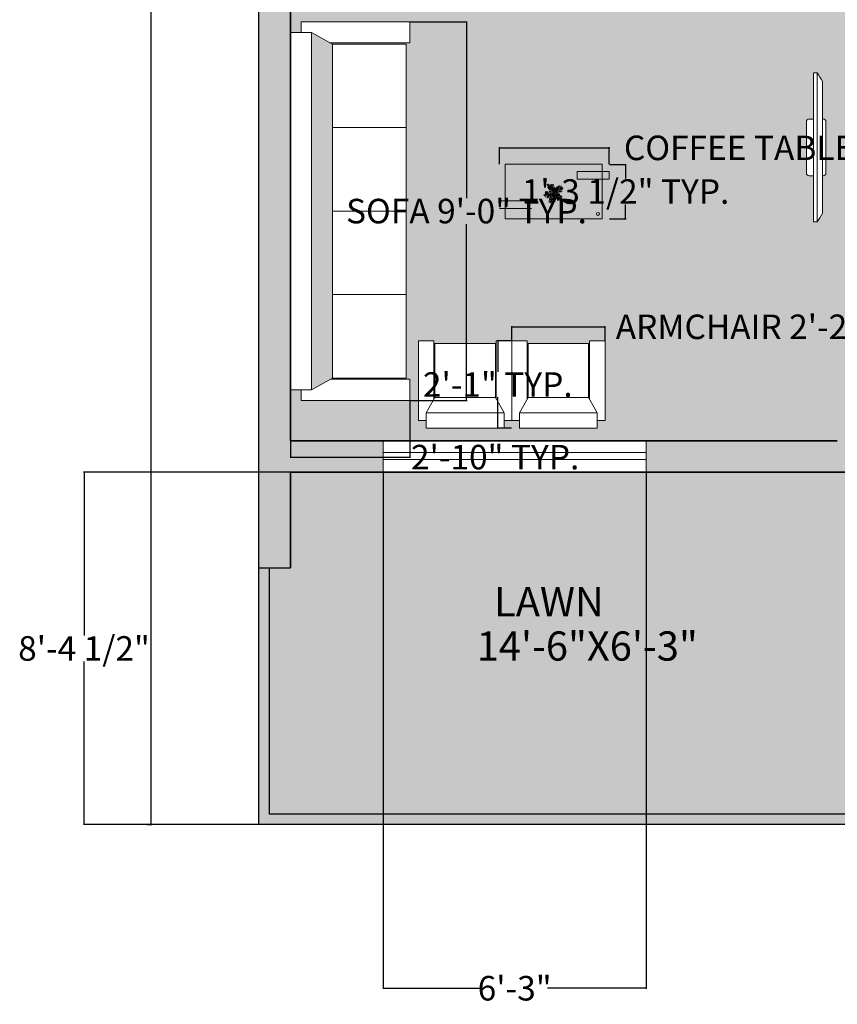
# Model space of a CAD drawing. Units: inches. Extents: x 1884 to 2398, y 474 to 1488.
# Tile 1 of 39: x 1884 to 2118, y 480 to 761. Entities that reach past the tile are written whole.
import ezdxf

# ---------------------------------------------------------------- set-up
doc = ezdxf.new("R2010")
doc.units = ezdxf.units.IN
doc.header["$MEASUREMENT"] = 0
doc.layers.get('0').update_dxf_attribs({"color": 250})
for name, color, linetype, lineweight in [('A-ANNO-DIMS', 2, 'Continuous', 18), ('A-AREA-IDEN', 7, 'Continuous', 18), ('A-EQPM', 8, 'Continuous', 18), ('A-FLOR-PATT', 254, 'Continuous', 13), ('A-FURN-PATT', 253, 'Continuous', 13), ('A-WALL-PATT', 250, 'Continuous', 13), ('C-PROP', 7, 'Continuous', 30), ('furniture', 8, 'Continuous', 18), ('L-PLNT', 73, 'Continuous', 18), ('L-TURF-PATT', 73, 'Continuous', 13), ('walls', 7, 'Continuous', 35), ('windows', 4, 'Continuous', 18)]:
    doc.layers.add(name, color=color, linetype=linetype, lineweight=lineweight)
doc.layers.add('A-FLOR-CASE-PATT', color=251, linetype='Continuous', lineweight=13, true_color=0x636466)
doc.styles.get("Standard").update_dxf_attribs({"font": 'arial.ttf'})
doc.dimstyles.get("Standard").update_dxf_attribs({"dimtxt": 7, "dimasz": 0.18, "dimexe": 0.18, "dimexo": 0.0625, "dimgap": 0.09, "dimtad": 0, "dimtih": 1, "dimtoh": 1, "dimzin": 0, "dimdsep": 46, "dimlunit": 3, "dimtxsty": 'Standard', "dimcen": 0.09, "dimadec": 0, "dimazin": 0, "dimtfac": 1, "dimtofl": 0, "dimtmove": 0, "dimatfit": 3, "dimfxl": 1, "dimtolj": 1, "dimtzin": 0, "dimarcsym": 0})

# ---------------------------------------------------------------- blocks, each defined once
blk = doc.blocks.new('*D2')
at = {"layer": 'A-ANNO-DIMS', "color": 0, "lineweight": -2, "transparency": 16777216}
for p, q in [((1920.51, 1406.88), (1921.96, 1406.88)), ((1921.78, 1406.7), (1921.78, 972.55)), ((1921.78, 531.06), (1921.78, 965.22)), ((1920.51, 530.88), (1921.96, 530.88))]:
    blk.add_line(p, q, dxfattribs=at)
at = {"layer": 'A-ANNO-DIMS', "color": 0, "lineweight": 100, "transparency": 16777216}
for points in [[(1921.75, 1406.7), (1921.81, 1406.7), (1921.78, 1406.88)], [(1921.75, 531.06), (1921.81, 531.06), (1921.78, 530.88)]]:
    blk.add_solid(points, dxfattribs=at)
at = {"layer": 'Defpoints', "color": 0, "lineweight": 100, "transparency": 16777216}
for p in [(1920.45, 1406.88), (1920.45, 530.88), (1921.78, 530.88)]:
    blk.add_point(p, dxfattribs=at)
at = {"layer": 'A-ANNO-DIMS', "color": 0, "transparency": 16777216, "insert": (1921.78, 968.88), "char_height": 7, "attachment_point": 5}
blk.add_mtext("\\A1;73'", dxfattribs=at)
blk = doc.blocks.new('tpoy')
at = {"layer": 'furniture'}
h = blk.add_hatch(color=256, dxfattribs=at)
h.dxf.hatch_style = 1
h.paths.add_polyline_path([(278.09, -251.06), (275.9, -251.06), (275.9, -258.19), (278.09, -258.19)])
h.paths.add_polyline_path([(278.09, -249.1), (275.9, -249.1), (275.9, -251.06), (278.09, -251.06)])
h.paths.add_polyline_path([(286.44, -271.28), (284.25, -271.28), (284.25, -278.76), (286.44, -278.76)])
h.paths.add_polyline_path([(286.44, -278.76), (284.25, -278.76), (284.25, -280.38), (286.44, -280.38)])
for p, q in [((275.9, -249.1), (278.09, -249.1)), ((275.9, -258.19), (275.9, -249.1)), ((278.09, -249.1), (278.09, -258.19)), ((273.86, -251.06), (273.86, -278.76)), ((289.38, -251.06), (273.86, -251.06)), ((289.38, -278.76), (289.38, -251.06)), ((278.09, -258.19), (275.9, -258.19)), ((284.25, -280.38), (284.25, -271.28)), ((286.44, -271.28), (286.44, -280.38)), ((273.86, -278.76), (289.38, -278.76))]:
    blk.add_line(p, q, dxfattribs=at)
blk.add_circle((288.03, -252.28), 0.401, dxfattribs=at)
blk = doc.blocks.new('*U20')
for p, q in [((-10.186, 53.64), (-13.084, 55.962)), ((0, 0), (-10.5, 57)), ((-9.099, 51.782), (-6.563, 55.962)), ((-47.498, 19.737), (-55.83, 18.344)), ((-40.615, 13.7), (-55.105, 10.913)), ((-31.5, 4.5), (-52.5, 25.5)), ((-33.37, 6.269), (-52.207, 5.34)), ((-48.585, 21.131), (-49.309, 29.026)), ((-28.299, 3.483), (-47.86, -5.805)), ((-43.513, 28.561), (-42.427, 15.558)), ((-38.442, 26.239), (-34.819, 7.663)), ((-21.416, 3.018), (-38.079, -8.128)), ((-35.544, 28.097), (-24.314, 3.947)), ((0, 0), (-31.5, 4.5)), ((-14.533, 2.09), (-30.834, 25.31)), ((-15.982, 2.09), (-30.11, -9.521)), ((-3.665, 19.273), (-27.574, 35.527)), ((-5.114, 28.097), (-24.676, 40.636)), ((-24.314, 23.917), (-2.941, 13.7)), ((0, 0), (-22.5, -19.5)), ((-7.288, 39.707), (-21.778, 46.673)), ((-6.563, 1.161), (-21.416, -8.128)), ((-20.691, 13.7), (-1.129, 4.876)), ((-8.737, 47.138), (-17.069, 52.711)), ((-7.65, 43.423), (-2.578, 49.46)), ((-5.839, 35.992), (4.667, 48.067)), ((-5.114, 27.632), (10.463, 46.673)), ((-2.941, 16.486), (8.652, 37.85)), ((-1.129, 6.734), (9.014, 26.704)), ((0, 0), (27, 9)), ((0, 0), (18, -22.5)), ((3.942, 1.625), (11.187, 24.381)), ((6.478, 1.625), (26.04, -8.592)), ((10.101, 3.483), (17.708, 26.239)), ((11.187, 3.483), (30.749, -5.805)), ((16.259, 5.805), (23.142, 31.348)), ((18.07, 5.805), (35.096, -3.483)), ((22.055, 7.198), (27.489, 32.277)), ((24.229, 7.663), (46.688, 1.625)), ((27, 9), (48, 36)), ((27.127, 9.056), (31.112, 35.992)), ((29.662, 12.307), (48.137, 6.269)), ((31.836, 30.883), (32.561, 16.486)), ((33.285, 16.486), (48.862, 10.913)), ((35.096, 32.741), (37.27, 22.524)), ((36.183, 19.737), (48.137, 17.88)), ((38.719, 34.134), (41.979, 28.561)), ((40.53, 25.775), (48.862, 24.846)), ((43.791, 29.954), (51.036, 30.883)), ((44.153, 36.456), (45.239, 32.741)), ((-17.431, -15.094), (-42.789, -18.809)), ((-28.299, -29.026), (-42.789, -31.348)), ((-24.314, -21.596), (-42.427, -22.06)), ((-30.834, -34.135), (-42.427, -35.528)), ((-34.457, -39.708), (-40.978, -42.494)), ((-26.849, -26.24), (-40.253, -25.775)), ((-22.5, -19.5), (-37.5, -45)), ((-32.646, -36.921), (-31.921, -44.352)), ((-15.257, -12.772), (-30.11, -12.772)), ((-29.023, -30.884), (-27.936, -43.887)), ((-25.038, -23.918), (-22.865, -45.281)), ((-20.691, -18.345), (-17.793, -44.352)), ((-6.563, -5.805), (-19.967, -9.985)), ((-17.069, -15.094), (-12.721, -40.172)), ((-13.446, -11.378), (-8.737, -32.741)), ((-9.461, -8.592), (-6.201, -23.453)), ((-4.752, -3.483), (-3.665, -14.629)), ((2.493, -3.019), (-1.491, -20.202)), ((1.769, -2.555), (24.229, -9.521)), ((5.029, -6.27), (2.131, -25.775)), ((9.014, -11.378), (3.58, -35.992)), ((14.085, -16.951), (6.478, -40.172)), ((7.565, -9.056), (32.198, -14.629)), ((18.07, -22.524), (8.289, -45.745)), ((12.274, -15.094), (36.907, -18.809)), ((20.244, -30.419), (15.897, -44.816)), ((16.259, -19.738), (36.183, -22.989)), ((18, -22.5), (27, -52.5)), ((18.433, -22.524), (40.53, -29.026)), ((19.157, -25.311), (38.719, -33.206)), ((22.78, -37.85), (19.519, -48.532)), ((21.331, -32.741), (39.081, -40.636)), ((22.78, -38.314), (34.372, -44.816)), ((24.591, -45.745), (23.142, -50.854)), ((24.591, -43.423), (30.749, -47.603)), ((26.764, -49.925), (28.213, -50.854))]:
    blk.add_line(p, q)
blk = doc.blocks.new('PLASMA-LARGE')
at = {"layer": 'furniture'}
for p, q in [((-7.26, 0), (7.26, 0)), ((-21, -2.5), (21, -2.5)), ((-21, -2.5), (-21, -3.5)), ((-18.61, -1), (18.61, -1)), ((-8, -1), (-8, -0.74)), ((8, -1), (8, -0.74)), ((21, -2.5), (21, -3.5)), ((-21, -3.5), (21, -3.5)), ((-8, -3.5), (-8, -4.76)), ((-7.26, -5.5), (7.26, -5.5)), ((8, -3.5), (8, -4.76))]:
    blk.add_line(p, q, dxfattribs=at)
for centre, radius, start, end in [((-7.26, -0.74), 0.744, 90, 180), ((7.26, -0.74), 0.744, 0, 90), ((-13.97, -11.05), 11.07, 114.7602, 129.4175), ((13.97, -11.05), 11.07, 50.5825, 65.2398), ((-7.26, -4.76), 0.744, 180, 270), ((7.26, -4.76), 0.744, 270, 0)]:
    blk.add_arc(centre, radius, start, end, dxfattribs=at)
blk = doc.blocks.new('FABRIC SOFA 4S')
at = {"layer": 'furniture'}
for p, q in [((3, 54), (34, 54)), ((3, 51), (3, 54)), ((34, 48), (34, 54)), ((0, -51), (0, 51)), ((6, 51), (0, 51)), ((6, -51), (6, 51)), ((12, 47.63), (6, 51)), ((11.14, 48), (34, 48)), ((33, 23.81), (12, 23.81)), ((33, 0), (12, 0)), ((33, -23.81), (12, -23.81)), ((6, -51), (12, -47.63)), ((11.54, -48), (34, -48)), ((34, -48), (34, -54)), ((6, -51), (0, -51)), ((3, -54), (3, -51)), ((3, -54), (34, -54))]:
    blk.add_line(p, q, dxfattribs=at)
blk.add_lwpolyline([(12, -47.63), (12, 47.63), (33, 47.63), (33, -47.63)], close=True, dxfattribs=at)
blk = doc.blocks.new('FABRIC SOFA 1S')
at = {"layer": 'furniture'}
for p, q in [((3, 18.12), (34, 18.12)), ((3, 15.12), (3, 18.12)), ((34, 12.12), (34, 18.12)), ((0, -15.12), (0, 15.12)), ((6, 15.12), (0, 15.12)), ((6, -15.12), (6, 15.12)), ((12, 11.75), (6, 15.12)), ((11.33, 12.12), (34, 12.12)), ((6, -15.12), (0, -15.12)), ((3, -18.12), (3, -15.12)), ((6, -15.12), (12, -11.75)), ((11.33, -12.12), (34, -12.12)), ((34, -12.12), (34, -18.12)), ((3, -18.12), (34, -18.12))]:
    blk.add_line(p, q, dxfattribs=at)
blk.add_lwpolyline([(12, -11.75), (12, 11.75), (33, 11.75), (33, -11.75)], close=True, dxfattribs=at)
blk = doc.blocks.new('*D29')
at = {"layer": 'A-ANNO-DIMS', "color": 0, "lineweight": -2, "transparency": 16777216}
for p, q in [((2024.65, 668.97), (2024.65, 673.08)), ((2024.83, 672.9), (2051.08, 672.9)), ((2051.26, 668.97), (2051.26, 673.08)), ((2051.26, 672.9), (2051.44, 672.9))]:
    blk.add_line(p, q, dxfattribs=at)
at = {"layer": 'A-ANNO-DIMS', "color": 0, "lineweight": 100, "transparency": 16777216}
for points in [[(2024.83, 672.93), (2024.83, 672.87), (2024.65, 672.9)], [(2051.08, 672.93), (2051.08, 672.87), (2051.26, 672.9)]]:
    blk.add_solid(points, dxfattribs=at)
at = {"layer": 'Defpoints', "color": 0, "lineweight": 100, "transparency": 16777216}
for p in [(2051.26, 672.9), (2024.65, 668.91), (2051.26, 668.91)]:
    blk.add_point(p, dxfattribs=at)
at = {"layer": 'A-ANNO-DIMS', "color": 0, "transparency": 16777216, "insert": (2108.66, 672.9), "char_height": 7, "attachment_point": 5}
blk.add_mtext('\\A1;ARMCHAIR 2\'-2 1/2" TYP.', dxfattribs=at)
blk = doc.blocks.new('*D30')
at = {"layer": 'A-ANNO-DIMS', "color": 0, "lineweight": -2, "transparency": 16777216}
for p, q in [((2024.59, 668.91), (2020.48, 668.91)), ((2020.66, 668.73), (2020.66, 660.04)), ((2020.66, 644.14), (2020.66, 652.83)), ((2024.59, 643.96), (2020.48, 643.96))]:
    blk.add_line(p, q, dxfattribs=at)
at = {"layer": 'A-ANNO-DIMS', "color": 0, "lineweight": 100, "transparency": 16777216}
for points in [[(2020.63, 668.73), (2020.69, 668.73), (2020.66, 668.91)], [(2020.63, 644.14), (2020.69, 644.14), (2020.66, 643.96)]]:
    blk.add_solid(points, dxfattribs=at)
at = {"layer": 'Defpoints', "color": 0, "lineweight": 100, "transparency": 16777216}
for p in [(2020.66, 668.91), (2024.65, 668.91), (2024.65, 643.96)]:
    blk.add_point(p, dxfattribs=at)
at = {"layer": 'A-ANNO-DIMS', "color": 0, "transparency": 16777216, "insert": (2020.66, 656.43), "char_height": 7, "attachment_point": 5}
blk.add_mtext('\\A1;2\'-1" TYP.', dxfattribs=at)
blk = doc.blocks.new('*D31')
at = {"layer": 'A-ANNO-DIMS', "color": 0, "lineweight": -2, "transparency": 16777216}
for p, q in [((1995.59, 759.92), (2011.91, 759.92)), ((2011.73, 759.74), (2011.73, 709.63)), ((2011.73, 652.1), (2011.73, 702.2)), ((1995.59, 651.92), (2011.91, 651.92))]:
    blk.add_line(p, q, dxfattribs=at)
at = {"layer": 'A-ANNO-DIMS', "color": 0, "lineweight": 100, "transparency": 16777216}
for points in [[(2011.7, 759.74), (2011.76, 759.74), (2011.73, 759.92)], [(2011.7, 652.1), (2011.76, 652.1), (2011.73, 651.92)]]:
    blk.add_solid(points, dxfattribs=at)
at = {"layer": 'Defpoints', "color": 0, "lineweight": 100, "transparency": 16777216}
for p in [(1995.53, 759.92), (2011.73, 759.92), (1995.53, 651.92)]:
    blk.add_point(p, dxfattribs=at)
at = {"layer": 'A-ANNO-DIMS', "color": 0, "transparency": 16777216, "insert": (2011.73, 705.92), "char_height": 7, "attachment_point": 5}
blk.add_mtext('\\A1;SOFA 9\'-0" TYP.', dxfattribs=at)
blk = doc.blocks.new('*D32')
at = {"layer": 'A-ANNO-DIMS', "color": 0, "lineweight": -2, "transparency": 16777216}
for p, q in [((1961.53, 651.85), (1961.53, 635.54)), ((1995.53, 651.85), (1995.53, 635.54)), ((1961.71, 635.72), (1995.35, 635.72)), ((1995.53, 635.72), (1995.71, 635.72))]:
    blk.add_line(p, q, dxfattribs=at)
at = {"layer": 'A-ANNO-DIMS', "color": 0, "lineweight": 100, "transparency": 16777216}
for points in [[(1961.71, 635.75), (1961.71, 635.69), (1961.53, 635.72)], [(1995.35, 635.75), (1995.35, 635.69), (1995.53, 635.72)]]:
    blk.add_solid(points, dxfattribs=at)
at = {"layer": 'Defpoints', "color": 0, "lineweight": 100, "transparency": 16777216}
for p in [(1961.53, 651.92), (1995.53, 651.92), (1995.53, 635.72)]:
    blk.add_point(p, dxfattribs=at)
at = {"layer": 'A-ANNO-DIMS', "color": 0, "transparency": 16777216, "insert": (2019.91, 635.72), "char_height": 7, "attachment_point": 5}
blk.add_mtext('\\A1;2\'-10" TYP.', dxfattribs=at)
blk = doc.blocks.new('*D33')
at = {"layer": 'A-ANNO-DIMS', "color": 0, "lineweight": -2, "transparency": 16777216}
for p, q in [((2021.15, 719.33), (2021.15, 724.14)), ((2021.33, 723.96), (2052.25, 723.96)), ((2052.43, 719.33), (2052.43, 724.14)), ((2052.43, 723.96), (2052.61, 723.96))]:
    blk.add_line(p, q, dxfattribs=at)
at = {"layer": 'A-ANNO-DIMS', "color": 0, "lineweight": 100, "transparency": 16777216}
for points in [[(2021.33, 723.99), (2021.33, 723.93), (2021.15, 723.96)], [(2052.25, 723.99), (2052.25, 723.93), (2052.43, 723.96)]]:
    blk.add_solid(points, dxfattribs=at)
at = {"layer": 'Defpoints', "color": 0, "lineweight": 100, "transparency": 16777216}
for p in [(2052.43, 723.96), (2021.15, 719.26), (2052.43, 719.26)]:
    blk.add_point(p, dxfattribs=at)
at = {"layer": 'A-ANNO-DIMS', "color": 0, "transparency": 16777216, "insert": (2120.18, 723.96), "char_height": 7, "attachment_point": 5}
blk.add_mtext('\\A1;COFFEE TABLE 2\'-7 1/2" TYP.', dxfattribs=at)
blk = doc.blocks.new('*D34')
at = {"layer": 'A-ANNO-DIMS', "color": 0, "lineweight": -2, "transparency": 16777216}
for p, q in [((2052.49, 719.26), (2057.3, 719.26)), ((2057.12, 719.08), (2057.12, 715.21)), ((2057.12, 703.92), (2057.12, 707.79)), ((2052.49, 703.74), (2057.3, 703.74))]:
    blk.add_line(p, q, dxfattribs=at)
at = {"layer": 'A-ANNO-DIMS', "color": 0, "lineweight": 100, "transparency": 16777216}
for points in [[(2057.09, 719.08), (2057.15, 719.08), (2057.12, 719.26)], [(2057.09, 703.92), (2057.15, 703.92), (2057.12, 703.74)]]:
    blk.add_solid(points, dxfattribs=at)
at = {"layer": 'Defpoints', "color": 0, "lineweight": 100, "transparency": 16777216}
for p in [(2052.43, 719.26), (2052.43, 703.74), (2057.12, 703.74)]:
    blk.add_point(p, dxfattribs=at)
at = {"layer": 'A-ANNO-DIMS', "color": 0, "transparency": 16777216, "insert": (2057.12, 711.5), "char_height": 7, "attachment_point": 5}
blk.add_mtext('\\A1;1\'-3 1/2" TYP.', dxfattribs=at)
blk = doc.blocks.new('*D55')
at = {"layer": 'A-ANNO-DIMS', "color": 0, "lineweight": -2, "transparency": 16777216}
for p, q in [((1988, 631.32), (1988, 484)), ((2062.95, 631.32), (2062.95, 484)), ((1988.18, 484.18), (2016.06, 484.18)), ((2062.77, 484.18), (2034.89, 484.18))]:
    blk.add_line(p, q, dxfattribs=at)
at = {"layer": 'A-ANNO-DIMS', "color": 0, "lineweight": 100, "transparency": 16777216}
for points in [[(1988.18, 484.21), (1988.18, 484.15), (1988, 484.18)], [(2062.77, 484.21), (2062.77, 484.15), (2062.95, 484.18)]]:
    blk.add_solid(points, dxfattribs=at)
at = {"layer": 'Defpoints', "color": 0, "lineweight": 100, "transparency": 16777216}
for p in [(1988, 631.38), (2062.95, 631.38), (2062.95, 484.18)]:
    blk.add_point(p, dxfattribs=at)
at = {"layer": 'A-ANNO-DIMS', "color": 0, "transparency": 16777216, "insert": (2025.48, 484.18), "char_height": 7, "attachment_point": 5}
blk.add_mtext('\\A1;6\'-3"', dxfattribs=at)
blk = doc.blocks.new('*D56')
at = {"layer": 'A-ANNO-DIMS', "color": 0, "lineweight": -2, "transparency": 16777216}
for p, q in [((1961.47, 631.38), (1902.43, 631.38)), ((1902.61, 631.2), (1902.61, 584.84)), ((1902.61, 531.06), (1902.61, 577.43)), ((1952.47, 530.88), (1902.43, 530.88))]:
    blk.add_line(p, q, dxfattribs=at)
at = {"layer": 'A-ANNO-DIMS', "color": 0, "lineweight": 100, "transparency": 16777216}
for points in [[(1902.58, 631.2), (1902.64, 631.2), (1902.61, 631.38)], [(1902.58, 531.06), (1902.64, 531.06), (1902.61, 530.88)]]:
    blk.add_solid(points, dxfattribs=at)
at = {"layer": 'Defpoints', "color": 0, "lineweight": 100, "transparency": 16777216}
for p in [(1902.61, 631.38), (1961.53, 631.38), (1952.53, 530.88)]:
    blk.add_point(p, dxfattribs=at)
at = {"layer": 'A-ANNO-DIMS', "color": 0, "transparency": 16777216, "insert": (1902.61, 581.13), "char_height": 7, "attachment_point": 5}
blk.add_mtext('\\A1;8\'-4 1/2"', dxfattribs=at)

msp = doc.modelspace()

# ---------------------------------------------------------------- hatches: boundary and pattern name
at = {"layer": 'A-FLOR-CASE-PATT'}
h = msp.add_hatch(color=256, dxfattribs=at)
h.dxf.hatch_style = 1
h.paths.add_polyline_path([(2101.332, 755.284), (2116.228, 755.284), (2116.228, 690.841), (2101.332, 690.841)])
h.paths.add_polyline_path([(2110.739, 702.864), (2111.75, 702.864, 0.0640419), (2113.267, 705.284), (2113.267, 716.011), (2113.526, 716.011, 0.4142136), (2114.278, 716.764), (2114.278, 731.439, 0.4142136), (2113.526, 732.192), (2113.267, 732.192), (2113.267, 742.92, 0.0640419), (2111.75, 745.339), (2110.739, 745.339), (2110.739, 732.192), (2109.469, 732.192, 0.4142136), (2108.716, 731.439), (2108.716, 716.764, 0.4142136), (2109.469, 716.011), (2110.739, 716.011)], flags=16)
at = {"layer": 'A-FLOR-PATT'}
h = msp.add_hatch(color=256, dxfattribs=at)
h.dxf.hatch_style = 1
h.paths.add_polyline_path([(2117.529, 815.801), (2126.529, 815.801), (2126.529, 880.382), (2117.529, 880.382), (2117.529, 892.385), (1961.529, 892.385), (1961.529, 756.915), (1964.529, 756.915), (1964.529, 759.915), (1995.529, 759.915), (1995.529, 753.915), (1972.862, 753.915), (1967.529, 756.915), (1967.529, 654.915), (1972.862, 657.915), (1995.529, 657.915), (1995.529, 651.915), (1964.529, 651.915), (1964.529, 654.915), (1961.529, 654.915), (1961.529, 640.385), (2117.529, 640.385), (2117.529, 646.578), (2126.529, 646.578), (2126.529, 676.183), (2117.529, 676.183)])
h.paths.add_polyline_path([(2012.246, 808.929), (2012.05, 810.185), (2032.542, 810.185), (2032.346, 808.929)], flags=16)
h.paths.add_polyline_path([(2010.381, 820.864), (1994.658, 820.864), (1994.658, 831.561), (1984.608, 833.132), (1984.608, 853.821), (1994.658, 855.391), (1994.658, 866.089), (2010.381, 866.089), (2011.951, 876.139), (2032.64, 876.139), (2034.211, 866.089), (2045.556, 866.089), (2047.127, 876.139), (2067.816, 876.139), (2069.386, 866.089), (2085.109, 866.089), (2085.109, 855.391), (2095.159, 853.821), (2095.159, 833.132), (2085.109, 831.561), (2085.109, 820.864), (2069.386, 820.864), (2067.816, 810.814), (2047.127, 810.814), (2045.556, 820.864), (2034.211, 820.864), (2032.64, 810.814), (2011.951, 810.814)], flags=16)
h.paths.add_polyline_path([(1982.724, 833.426), (1982.724, 853.526), (1983.98, 853.723), (1983.98, 833.23)], flags=16)
h.paths.add_polyline_path([(1994.529, 753.54), (1994.529, 658.29), (1973.529, 658.29), (1973.529, 753.54)], flags=16)
h.paths.add_polyline_path([(2084.486, 843.527), (2084.592, 843.502), (2084.681, 843.487), (2084.813, 843.477), (2084.913, 843.477), (2084.669, 843.482), (2084.336, 843.565), (2084.116, 843.617), (2083.8, 843.686), (2083.105, 843.827), (2082.836, 843.874), (2083.604, 843.729), (2084.206, 843.597)], flags=0)
h.paths.add_polyline_path([(2047.421, 808.929), (2047.225, 810.185), (2067.718, 810.185), (2067.521, 808.929)], flags=16)
h.paths.add_polyline_path([(2066.01, 849.505), (2066.429, 849.687), (2066.798, 849.882), (2067.129, 850.085), (2067.43, 850.293), (2067.711, 850.502), (2068.176, 850.856), (2068.689, 851.205), (2069.305, 851.531), (2070.015, 851.784), (2070.844, 851.944), (2071.081, 851.956), (2070.629, 851.902), (2070.212, 851.822), (2069.827, 851.717), (2069.471, 851.59), (2069.139, 851.443), (2068.828, 851.279), (2068.534, 851.1), (2068.254, 850.909), (2067.983, 850.709), (2067.502, 850.343), (2066.951, 849.962), (2066.224, 849.579)], flags=0)
h.paths.add_polyline_path([(2059.423, 853.221), (2059.827, 853.278), (2060.171, 853.358), (2060.465, 853.463), (2060.714, 853.589), (2060.926, 853.736), (2061.107, 853.902), (2061.258, 854.086), (2061.377, 854.284), (2061.462, 854.495), (2061.514, 854.715), (2061.53, 854.943), (2061.508, 855.176), (2061.449, 855.411), (2061.352, 855.646), (2061.224, 855.882), (2061.07, 856.117), (2060.9, 856.353), (2060.719, 856.588), (2060.406, 856.993), (2060.103, 857.424), (2059.858, 857.888), (2059.691, 858.467), (2059.836, 859.091), (2060.305, 859.532), (2060.844, 859.798), (2061.513, 859.935), (2062.253, 859.905), (2062.483, 859.849), (2062.078, 859.912), (2061.695, 859.928), (2061.336, 859.899), (2061.005, 859.831), (2060.703, 859.729), (2060.437, 859.597), (2060.208, 859.441), (2060.021, 859.265), (2059.879, 859.075), (2059.785, 858.874), (2059.737, 858.664), (2059.73, 858.447), (2059.761, 858.224), (2059.827, 857.996), (2059.923, 857.765), (2060.047, 857.53), (2060.193, 857.295), (2060.359, 857.06), (2060.537, 856.824), (2060.867, 856.399), (2061.171, 855.978), (2061.422, 855.518), (2061.567, 854.943), (2061.41, 854.272), (2060.947, 853.707), (2060.335, 853.397), (2059.649, 853.236)], flags=0)
h.paths.add_polyline_path([(2050.778, 859.745), (2051.07, 859.87), (2051.295, 860.017), (2051.467, 860.183), (2051.594, 860.365), (2051.679, 860.56), (2051.726, 860.763), (2051.739, 860.971), (2051.722, 861.18), (2051.677, 861.387), (2051.609, 861.587), (2051.521, 861.779), (2051.421, 861.962), (2051.312, 862.138), (2051.203, 862.307), (2050.966, 862.68), (2050.793, 863.193), (2051.021, 863.699), (2051.483, 864.018), (2052.09, 864.138), (2052.773, 864.157), (2053.007, 864.142), (2052.603, 864.152), (2052.258, 864.142), (2051.965, 864.113), (2051.716, 864.064), (2051.504, 863.995), (2051.322, 863.907), (2051.17, 863.802), (2051.048, 863.682), (2050.954, 863.55), (2050.891, 863.408), (2050.856, 863.259), (2050.851, 863.105), (2050.876, 862.948), (2050.929, 862.791), (2051.005, 862.633), (2051.098, 862.472), (2051.203, 862.307), (2051.312, 862.138), (2051.556, 861.742), (2051.751, 861.167), (2051.712, 860.535), (2051.398, 860.085), (2050.949, 859.79)], flags=0)
h.paths.add_polyline_path([(2022.768, 719.264), (2050.461, 719.264), (2050.461, 717.226), (2052.426, 717.226), (2052.426, 715.033), (2050.461, 715.033), (2050.461, 703.738), (2022.768, 703.738)], flags=16)
h.paths.add_polyline_path([(2012.246, 878.023), (2032.346, 878.023), (2032.542, 876.767), (2012.05, 876.767)], flags=16)
h.paths.add_polyline_path([(2035.324, 713.103), (2035.342, 713.294), (2035.192, 713.202)], flags=0)
h.paths.add_polyline_path([(2036.484, 711.63), (2036.583, 711.849), (2036.39, 711.898)], flags=0)
h.paths.add_polyline_path([(2036.074, 712.744), (2035.993, 712.481), (2035.724, 712.516), (2035.794, 712.726)], flags=0)
h.paths.add_polyline_path([(2035.846, 710.909), (2035.753, 710.958), (2035.702, 710.88)], flags=0)
h.paths.add_polyline_path([(2037.818, 712.019), (2037.948, 712.06), (2037.987, 712.161), (2037.815, 712.02)], flags=0)
h.paths.add_polyline_path([(2038.451, 709.517), (2038.464, 709.428), (2038.586, 709.442)], flags=0)
h.paths.add_polyline_path([(2037.805, 709.806), (2037.818, 709.807), (2037.804, 709.823)], flags=0)
h.paths.add_polyline_path([(2036.7, 711.245), (2036.698, 711.236), (2036.813, 711.211)], flags=0)
h.paths.add_polyline_path([(2035.928, 708.897), (2035.668, 708.871), (2035.706, 708.667)], flags=0)
h.paths.add_polyline_path([(2036.414, 710.976), (2035.932, 709.859), (2036.792, 710.484), (2036.5, 710.934)], flags=0)
h.paths.add_polyline_path([(2038.298, 712.115), (2038.499, 712.058), (2038.612, 712.269), (2038.39, 712.332)], flags=0)
h.paths.add_polyline_path([(2047.421, 878.023), (2067.521, 878.023), (2067.718, 876.767), (2047.225, 876.767)], flags=16)
h.paths.add_polyline_path([(2049.647, 705.093, -1), (2048.845, 705.093, -1)], flags=0)
h.paths.add_polyline_path([(2095.787, 853.723), (2097.043, 853.526), (2097.043, 833.426), (2095.787, 833.23)], flags=16)
h.paths.add_polyline_path([(2110.739, 745.339), (2111.75, 745.339, -0.0640419), (2113.267, 742.92), (2113.267, 732.192), (2113.526, 732.192, -0.4142136), (2114.278, 731.439), (2114.278, 716.764, -0.4142136), (2113.526, 716.011), (2113.267, 716.011), (2113.267, 705.284, -0.0640419), (2111.75, 702.864), (2110.739, 702.864), (2110.739, 716.011), (2109.469, 716.011, -0.4142136), (2108.716, 716.764), (2108.716, 731.439, -0.4142136), (2109.469, 732.192), (2110.739, 732.192)], flags=16)
h.paths.add_polyline_path([(1998.045, 668.909), (2002.449, 668.909), (2002.449, 652.273), (2002.724, 652.763), (2002.724, 668.175), (2019.972, 668.175), (2019.972, 652.763), (2020.247, 652.273), (2020.247, 668.909), (2024.651, 668.909), (2029.055, 668.909), (2029.055, 652.273), (2029.33, 652.763), (2029.33, 668.175), (2046.578, 668.175), (2046.578, 652.763), (2046.853, 652.273), (2046.853, 668.909), (2051.257, 668.909), (2051.257, 646.157), (2049.055, 646.157), (2049.055, 643.955), (2026.853, 643.955), (2026.853, 646.157), (2024.651, 646.157), (2022.449, 646.157), (2022.449, 643.955), (2000.247, 643.955), (2000.247, 646.157), (1998.045, 646.157)], flags=16)
h.paths.add_polyline_path([(2342.529, 1247.885), (2265.892, 1247.885), (2230.029, 1247.885), (2209.755, 1247.885), (2168.6, 1247.885), (2168.6, 1104.929), (2158.029, 1104.929), (2158.029, 1079.411), (2168.6, 1079.411), (2168.6, 1062.466), (2342.529, 1062.466), (2342.529, 1093.809)])
h.paths.add_polyline_path([(2215.03, 1153.876), (2215.03, 1164.739), (2187.559, 1164.739), (2187.442, 1152.641), (2173.568, 1152.641), (2173.684, 1164.739), (2173.684, 1218.739), (2173.801, 1230.837), (2187.675, 1230.837), (2187.559, 1218.739), (2215.03, 1218.739), (2215.03, 1225.879), (2245.053, 1225.879), (2245.053, 1153.876)], flags=16)
h.paths.add_polyline_path([(2192.147, 1164.797), (2184.963, 1174.54), (2184.915, 1174.54), (2176.755, 1174.54), (2176.755, 1190.363), (2184.915, 1190.363), (2184.915, 1196.819), (2176.755, 1196.819), (2176.755, 1212.641), (2184.915, 1212.641), (2184.915, 1174.606), (2184.963, 1174.54), (2192.147, 1174.54)], flags=0)
h.paths.add_polyline_path([(2184.971, 1158.364, -1), (2176.039, 1158.364, -1)], flags=0)
h.paths.add_polyline_path([(2335.555, 1161.985), (2335.555, 1175.132), (2334.285, 1175.132, -0.4142136), (2333.533, 1175.885), (2333.533, 1190.56, -0.4142136), (2334.285, 1191.313), (2335.555, 1191.313), (2335.555, 1204.46), (2336.567, 1204.46, -0.0640419), (2338.083, 1202.04), (2338.083, 1191.313), (2338.342, 1191.313, -0.4142136), (2339.095, 1190.56), (2339.095, 1175.885, -0.4142136), (2338.342, 1175.132), (2338.083, 1175.132), (2338.083, 1164.405, -0.0640419), (2336.567, 1161.985)], flags=16)
h.paths.add_polyline_path([(2176.155, 1224.462, -1), (2185.087, 1224.462, -1)], flags=0)
h.paths.add_polyline_path([(2158.029, 1276.197), (2158.029, 1322.885), (2148.233, 1322.885), (2092.029, 1322.885), (1961.529, 1322.885), (1961.529, 1166.885), (2116.005, 1166.885), (2116.005, 1157.885), (2152.638, 1157.885), (2152.638, 1166.885), (2158.029, 1166.885)])
h.paths.add_polyline_path([(2006.352, 1204.245), (2006.352, 1215.108), (1978.881, 1215.108), (1978.764, 1203.01), (1964.89, 1203.01), (1965.006, 1215.108), (1965.006, 1269.108), (1965.123, 1281.207), (1978.997, 1281.207), (1978.881, 1269.108), (2006.352, 1269.108), (2006.352, 1276.248), (2036.375, 1276.248), (2036.375, 1204.245)], flags=16)
h.paths.add_polyline_path([(1983.469, 1215.166), (1976.285, 1224.909), (1976.237, 1224.909), (1968.077, 1224.909), (1968.077, 1240.732), (1976.237, 1240.732), (1976.237, 1247.188), (1968.077, 1247.188), (1968.077, 1263.011), (1976.237, 1263.011), (1976.237, 1224.975), (1976.285, 1224.909), (1983.469, 1224.909)], flags=0)
h.paths.add_polyline_path([(1976.293, 1208.733, -1), (1967.361, 1208.733, -1)], flags=0)
h.paths.add_polyline_path([(1967.477, 1274.832, -1), (1976.41, 1274.832, -1)], flags=0)
h.paths.add_polyline_path([(2152.587, 1223.485), (2152.587, 1236.632), (2151.317, 1236.632, -0.4142136), (2150.564, 1237.385), (2150.564, 1252.06, -0.4142136), (2151.317, 1252.813), (2152.587, 1252.813), (2152.587, 1265.959), (2153.598, 1265.959, -0.0640419), (2155.115, 1263.54), (2155.115, 1252.813), (2155.374, 1252.813, -0.4142136), (2156.126, 1252.06), (2156.126, 1237.385, -0.4142136), (2155.374, 1236.632), (2155.115, 1236.632), (2155.115, 1225.904, -0.0640419), (2153.598, 1223.485)], flags=16)
h.paths.add_polyline_path([(2250.676, 1161.101), (2322.077, 1161.101), (2322.077, 1173.886), (2250.676, 1173.886)], flags=24)
h.paths.add_polyline_path([(2255.61, 1173.712), (2320.136, 1173.712), (2320.136, 1186.659), (2255.61, 1186.659)], flags=24)
h.paths.add_polyline_path([(2053.687, 1230.837), (2125.089, 1230.837), (2125.089, 1243.622), (2053.687, 1243.622)], flags=24)
h.paths.add_polyline_path([(2058.622, 1243.448), (2123.147, 1243.448), (2123.147, 1256.395), (2058.622, 1256.395)], flags=24)
at = {"layer": 'A-FURN-PATT'}
h = msp.add_hatch(color=256, dxfattribs=at)
h.dxf.hatch_style = 1
h.paths.add_polyline_path([(2050.461, 715.033), (2043.335, 715.033), (2043.335, 717.226), (2050.461, 717.226), (2050.461, 719.264), (2022.768, 719.264), (2022.768, 708.874), (2030.239, 708.874), (2030.239, 706.68), (2022.768, 706.68), (2022.768, 703.738), (2050.461, 703.738)])
h.paths.add_polyline_path([(2038.607, 712.27), (2038.612, 712.269), (2038.615, 712.273)], flags=16)
h.paths.add_polyline_path([(2036.679, 711.078), (2035.246, 710.788), (2035.256, 710.805), (2035.27, 710.793), (2036.679, 711.078), (2036.195, 712.449), (2036.185, 712.456), (2036.193, 712.455), (2036.679, 711.078), (2036.813, 711.189), (2036.819, 711.21), (2036.835, 711.207), (2036.679, 711.078), (2037.451, 710.216), (2037.462, 710.218), (2037.465, 710.201)], flags=16)
h.paths.add_polyline_path([(2049.647, 705.093, -1), (2048.845, 705.093, -1)], flags=16)
at = {"layer": 'A-WALL-PATT'}
h = msp.add_hatch(color=256, dxfattribs=at)
h.dxf.hatch_style = 1
h.paths.add_polyline_path([(2351.529, 837.963), (2342.529, 837.963), (2342.529, 813.478), (2351.529, 813.478)])
h.paths.add_polyline_path([(2351.529, 782.175), (2342.529, 782.175), (2342.529, 778.966), (2238.447, 778.966), (2238.447, 769.966), (2351.529, 769.966)])
h.paths.add_polyline_path([(2351.529, 914.773), (2342.529, 914.773), (2342.529, 901.966), (2222.529, 901.966), (2222.529, 908.236), (2213.529, 908.236), (2213.529, 901.966), (2198.529, 901.966), (2198.529, 892.966), (2198.529, 815.857), (2203.029, 815.857), (2203.029, 892.966), (2342.529, 892.966), (2342.529, 869.555), (2346.047, 869.555), (2351.529, 869.555), (2351.529, 880.385)])
h.paths.add_polyline_path([(2208.948, 778.966), (2203.029, 778.966), (2203.029, 782.647), (2198.529, 782.647), (2198.529, 779.109), (2193.526, 779.109), (2193.526, 769.966), (2198.529, 769.966), (2208.948, 769.966)])
h.paths.add_polyline_path([(2126.529, 815.801), (2117.529, 815.801), (2117.529, 676.183), (2126.529, 676.183), (2126.529, 769.966), (2132.515, 769.966), (2132.515, 778.664), (2126.529, 778.664)])
h.paths.add_polyline_path([(2135.996, 901.385), (2009.529, 901.385), (2009.529, 929.544), (2000.529, 929.544), (2000.529, 892.385), (2117.529, 892.385), (2117.529, 880.382), (2126.529, 880.382), (2126.529, 892.385), (2135.996, 892.385)])
h.paths.add_polyline_path([(2198.529, 901.385), (2185.2, 901.385), (2185.2, 892.385), (2198.529, 892.385), (2198.529, 892.966)])
h.paths.add_polyline_path([(1961.529, 892.385), (1965.143, 892.385), (1965.143, 901.385), (1952.529, 901.385), (1952.529, 604.13), (1961.529, 604.13), (1961.529, 631.385), (1988.002, 631.385), (1988.002, 640.385), (1961.529, 640.385)])
h.paths.add_polyline_path([(1955.529, 604.13), (1952.529, 604.13), (1952.529, 530.885), (2126.529, 530.885), (2126.529, 533.885), (1955.529, 533.885)])
h.paths.add_polyline_path([(2396.529, 604.13), (2393.529, 604.13), (2393.529, 533.885), (2126.529, 533.885), (2126.529, 530.885), (2396.529, 530.885)])
h.paths.add_polyline_path([(2396.529, 779.322), (2387.529, 779.322), (2387.529, 604.13), (2396.529, 604.13)])
h = msp.add_hatch(color=256, dxfattribs=at)
h.dxf.hatch_style = 1
h.paths.add_polyline_path([(2126.529, 646.578), (2117.529, 646.578), (2117.529, 640.385), (2062.952, 640.385), (2062.952, 631.385), (2126.529, 631.385)])
at = {"layer": 'L-TURF-PATT'}
h = msp.add_hatch(color=256, dxfattribs=at)
h.dxf.hatch_style = 1
h.paths.add_polyline_path([(2126.529, 607.943), (2117.364, 607.943), (2117.364, 631.385), (1961.529, 631.385), (1961.529, 604.13), (1955.529, 604.13), (1955.529, 533.885), (2126.529, 533.885)])
h = msp.add_hatch(color=256, dxfattribs=at)
h.dxf.hatch_style = 1
h.paths.add_polyline_path([(2120.392, 631.385), (2117.364, 631.385), (2117.364, 607.943), (2126.529, 607.943), (2126.529, 611.008), (2120.392, 611.008)])
h.paths.add_polyline_path([(2126.529, 631.385), (2120.392, 631.385), (2120.392, 611.008), (2126.529, 611.008)], flags=17)

# ---------------------------------------------------------------- linework, layer by layer
at = {"layer": 'C-PROP'}
for p, q in [((1952.529, 530.885), (1952.529, 901.385)), ((1952.529, 604.13), (1961.529, 604.13)), ((1955.529, 533.885), (1955.529, 604.13)), ((2393.529, 533.885), (1955.529, 533.885)), ((2396.529, 530.885), (1952.529, 530.885))]:
    msp.add_line(p, q, dxfattribs=at)
at = {"layer": 'walls'}
for p, q in [((1961.529, 640.385), (1961.529, 892.385)), ((1961.529, 640.385), (2117.529, 640.385)), ((1961.529, 604.13), (1961.529, 631.385)), ((1961.529, 631.385), (2126.529, 631.385))]:
    msp.add_line(p, q, dxfattribs=at)
at = {"layer": 'windows'}
for p, q in [((1988.002, 640.385), (1988.002, 631.385)), ((2062.952, 640.385), (1988.002, 640.385)), ((1988.002, 640.385), (1988.002, 637.025)), ((2062.952, 631.385), (2062.952, 640.385)), ((1988.002, 637.025), (2062.952, 637.025)), ((2062.952, 635.073), (1988.002, 635.073)), ((2062.952, 637.025), (2062.952, 635.073)), ((1988.002, 631.385), (2062.952, 631.385))]:
    msp.add_line(p, q, dxfattribs=at)

# ---------------------------------------------------------------- block references
at = {"layer": 'A-EQPM', "xscale": -1.011294184530666, "yscale": 1.011294184530666, "zscale": 1.011294184530666, "rotation": 270}
msp.add_blockref('PLASMA-LARGE', (2114.278, 724.102), dxfattribs=at)
at = {"layer": 'furniture'}
msp.add_blockref('FABRIC SOFA 4S', (1961.529, 705.915), dxfattribs=at)
at = {"layer": 'furniture', "rotation": 270}
msp.add_blockref('tpoy', (2301.523, 993.122), dxfattribs=at)
at = {"layer": 'furniture', "xscale": -0.7339463821036302, "yscale": 0.7339463821036302, "zscale": 0.7339463821036302}
for p, rotation in [((2011.348, 643.955), 270), ((2037.954, 643.955), 269.9999999999993)]:
    msp.add_blockref('FABRIC SOFA 1S', p, dxfattribs=dict(at, rotation=rotation))
at = {"layer": 'L-PLNT', "xscale": 0.0510892351028333, "yscale": 0.0510892351028333, "zscale": 0.0510892351028333, "rotation": 90.98387132377816}
msp.add_blockref('*U20', (2036.679, 711.078), dxfattribs=at)

# ---------------------------------------------------------------- texts
at = {"layer": 'A-AREA-IDEN'}
for s, height, p in [('LAWN', 8.3413, (2019.597, 590.279)), ('14\'-6"X6\'-3"', 8.34125, (2014.635, 577.646))]:
    msp.add_text(s, height=height, dxfattribs=at).set_placement(p)

# ---------------------------------------------------------------- dimensions: what is measured, and where the dimension line sits
at = {"layer": 'A-ANNO-DIMS'}
for base, p1, p2, override, picture, middle in [((1921.782, 530.885), (1920.445, 1406.885), (1920.445, 530.885), {"dimclrd": 0, "dimclre": 0, "dimclrt": 0}, '*D2', (1921.782, 968.885)), ((1902.612, 631.385), (1952.529, 530.885), (1961.529, 631.385), {"dimdec": 1, "dimlfac": 1, "dimrnd": 0, "dimzin": 1, "dimdsep": 46, "dimlunit": 4, "dimfrac": 2}, '*D56', (1902.612, 581.135))]:
    dim = msp.add_linear_dim(base=base, p1=p1, p2=p2, angle=90, dimstyle='Standard', override=override, dxfattribs=at)
    dim.commit()
    dim.dimension.update_dxf_attribs({"geometry": picture, "text_midpoint": middle})
for base, p1, p2, angle, text, picture, middle in [((2011.729, 759.915), (1995.529, 651.915), (1995.529, 759.915), 90, 'SOFA <> TYP.', '*D31', (2011.729, 705.915)), ((2057.118, 703.738), (2052.426, 719.264), (2052.426, 703.738), 270, '<> TYP.', '*D34', (2057.118, 711.501)), ((2020.66, 668.909), (2024.651, 643.955), (2024.651, 668.909), 90, '<> TYP.', '*D30', (2020.66, 656.432))]:
    dim = msp.add_linear_dim(base=base, p1=p1, p2=p2, angle=angle, text=text, dimstyle='Standard', override={"dimdec": 1, "dimlfac": 1, "dimrnd": 0, "dimzin": 1, "dimdsep": 46, "dimlunit": 4, "dimfrac": 2}, dxfattribs=at)
    dim.commit()
    dim.dimension.update_dxf_attribs({"geometry": picture, "text_midpoint": middle})
for base, p1, p2, text, picture, middle in [((2052.426, 723.955), (2021.148, 719.264), (2052.426, 719.264), 'COFFEE TABLE <> TYP.', '*D33', (2120.182, 723.955)), ((2051.257, 672.9), (2024.651, 668.909), (2051.257, 668.909), 'ARMCHAIR <> TYP.', '*D29', (2108.656, 672.9)), ((1995.529, 635.715), (1961.529, 651.915), (1995.529, 651.915), '<> TYP.', '*D32', (2019.912, 635.715))]:
    dim = msp.add_linear_dim(base=base, p1=p1, p2=p2, text=text, dimstyle='Standard', override={"dimdec": 1, "dimlfac": 1, "dimrnd": 0, "dimzin": 1, "dimdsep": 46, "dimlunit": 4, "dimfrac": 2}, dxfattribs=at)
    dim.commit()
    dim.dimension.update_dxf_attribs({"geometry": picture, "text_midpoint": middle})
dim = msp.add_linear_dim(base=(2062.9524, 484.1847), p1=(1988.0019, 631.3847), p2=(2062.9524, 631.3847), dimstyle='Standard', override={"dimdec": 1, "dimlfac": 1, "dimrnd": 0, "dimzin": 1, "dimdsep": 46, "dimlunit": 4, "dimfrac": 2}, dxfattribs=at)
dim.commit()
dim.dimension.update_dxf_attribs({"geometry": '*D55', "text_midpoint": (2025.4772, 484.1847)})

doc.saveas('drawing.dxf')
